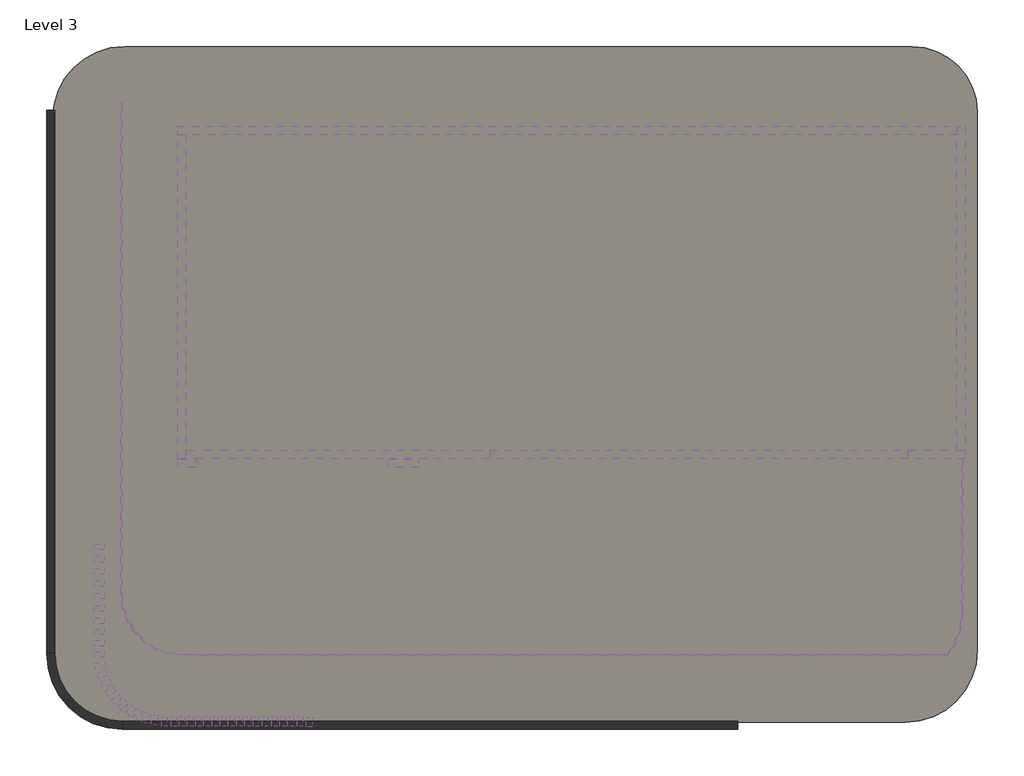
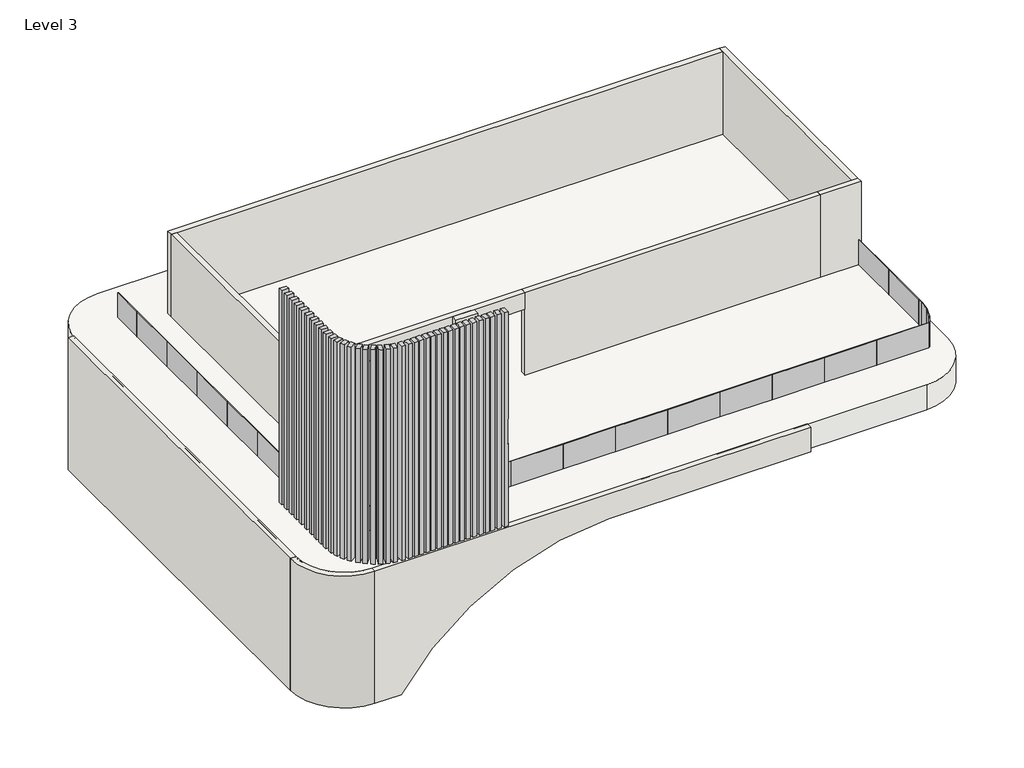
# One storey: 38 columns, 31 plates, 11 walls, 1 slab.
"""IFC4 building model written with IfcOpenShell, lengths in millimetres."""

from ifc_helpers import new_model, si_unit, point, frame, frame_2d, origin, place, context, project, spatial, polyline, circle_curve, trimmed, segment, composite_curve, outline, extrude, faceted_brep, transform, mapped, element, save
from components import wood_timber_column_6_x_10_a3b0a8a3, system_panel_glazed_95be5de7, system_panel_glazed_8df4d628, system_panel_glazed_8746fe8c, system_panel_glazed_e5de8428, system_panel_glazed_70ef586e, system_panel_glazed_2e848b93, system_panel_glazed_d6f392a9, system_panel_glazed_76d2efde, system_panel_glazed_ca107f82, system_panel_glazed_2060cbb7, system_panel_glazed_2c748f7c

model = new_model("IFC4")

# Units and contexts
model_context = context("Model", 3, world=origin())
ifc_project = project(units=[si_unit("LENGTHUNIT", "METRE", prefix="MILLI")], contexts=[model_context])

# Site, building, storey
site = spatial("IfcSite", under=ifc_project)
building = spatial("IfcBuilding", under=site)
storey = spatial("IfcBuildingStorey", under=building, Name="Level 3", Elevation=6096.0)

# Columns
placement = place(None, origin())
element("IfcColumn", 1, ObjectType="Wood Timber Column : 6 x 10", at=placement, inside=storey, context=model_context, shape_type="Brep", body=[
    faceted_brep([(-12385.9213551, -2400.8102607, 7931.15), (-12525.6213551, -2400.8102607, 7931.15), (-12525.6213551, -2159.5102607, 7931.15), (-12385.9213551, -2159.5102607, 7931.15), (-12385.9213551, -2400.8102607, 10979.15), (-12401.7963551, -2400.8102607, 10979.15), (-12401.7963551, -2400.8102607, 11893.55), (-12385.9213551, -2400.8102607, 11893.55), (-12385.9213551, -2400.8102607, 15855.95), (-12525.6213551, -2400.8102607, 15855.95), (-12525.6213551, -2159.5102607, 15855.95), (-12385.9213551, -2159.5102607, 15855.95), (-12385.9213551, -2284.9227607, 11893.55), (-12385.9213551, -2284.9227607, 10979.15), (-12401.7963551, -2284.9227607, 11893.55), (-12401.7963551, -2284.9227607, 10979.15)], [[[0, 1, 2, 3]], [[1, 0, 4, 5, 6, 7, 8, 9]], [[2, 1, 9, 10]], [[3, 2, 10, 11]], [[0, 3, 11, 8, 7, 12, 13, 4]], [[9, 8, 11, 10]], [[14, 15, 13, 12]], [[14, 12, 7, 6]], [[15, 14, 6, 5]], [[13, 15, 5, 4]]]),
])
wood_timber_column_6_x_10_shape = wood_timber_column_6_x_10_a3b0a8a3(model_context)
element("IfcColumn", 2, ObjectType="Wood Timber Column : 6 x 10", at=placement, inside=storey, context=model_context, shape_type="MappedRepresentation", body=[
    mapped(wood_timber_column_6_x_10_shape, transform((-12684.3713551, -2267.4602607, 0.0), x_axis=(1.0, 0.0, 0.0), y_axis=(0.0, 1.0, 0.0), z_axis=(0.0, 0.0, 1.0))),
])
element("IfcColumn", 3, ObjectType="Wood Timber Column : 6 x 10", at=placement, inside=storey, context=model_context, shape_type="MappedRepresentation", body=[
    mapped(wood_timber_column_6_x_10_shape, transform((-12912.9713551, -2267.4602607, 0.0), x_axis=(1.0, 0.0, 0.0), y_axis=(0.0, 1.0, 0.0), z_axis=(0.0, 0.0, 1.0))),
])
element("IfcColumn", 4, ObjectType="Wood Timber Column : 6 x 10", at=placement, inside=storey, context=model_context, shape_type="MappedRepresentation", body=[
    mapped(wood_timber_column_6_x_10_shape, transform((-13116.1713551, -2267.4602607, 0.0), x_axis=(1.0, 0.0, 0.0), y_axis=(0.0, 1.0, 0.0), z_axis=(0.0, 0.0, 1.0))),
])
element("IfcColumn", 5, ObjectType="Wood Timber Column : 6 x 10", at=placement, inside=storey, context=model_context, shape_type="MappedRepresentation", body=[
    mapped(wood_timber_column_6_x_10_shape, transform((-13319.3713551, -2267.4602607, 0.0), x_axis=(1.0, 0.0, 0.0), y_axis=(0.0, 1.0, 0.0), z_axis=(0.0, 0.0, 1.0))),
])
element("IfcColumn", 6, ObjectType="Wood Timber Column : 6 x 10", at=placement, inside=storey, context=model_context, shape_type="MappedRepresentation", body=[
    mapped(wood_timber_column_6_x_10_shape, transform((-13547.9713551, -2267.4602607, 0.0), x_axis=(1.0, 0.0, 0.0), y_axis=(0.0, 1.0, 0.0), z_axis=(0.0, 0.0, 1.0))),
])
element("IfcColumn", 7, ObjectType="Wood Timber Column : 6 x 10", at=placement, inside=storey, context=model_context, shape_type="MappedRepresentation", body=[
    mapped(wood_timber_column_6_x_10_shape, transform((-13776.5713551, -2267.4602607, 0.0), x_axis=(1.0, 0.0, 0.0), y_axis=(0.0, 1.0, 0.0), z_axis=(0.0, 0.0, 1.0))),
])
element("IfcColumn", 8, ObjectType="Wood Timber Column : 6 x 10", at=placement, inside=storey, context=model_context, shape_type="MappedRepresentation", body=[
    mapped(wood_timber_column_6_x_10_shape, transform((-13979.7713551, -2267.4602607, 0.0), x_axis=(1.0, 0.0, 0.0), y_axis=(0.0, 1.0, 0.0), z_axis=(0.0, 0.0, 1.0))),
])
element("IfcColumn", 9, ObjectType="Wood Timber Column : 6 x 10", at=placement, inside=storey, context=model_context, shape_type="MappedRepresentation", body=[
    mapped(wood_timber_column_6_x_10_shape, transform((-14182.9713551, -2267.4602607, 0.0), x_axis=(1.0, 0.0, 0.0), y_axis=(0.0, 1.0, 0.0), z_axis=(0.0, 0.0, 1.0))),
])
element("IfcColumn", 10, ObjectType="Wood Timber Column : 6 x 10", at=placement, inside=storey, context=model_context, shape_type="MappedRepresentation", body=[
    mapped(wood_timber_column_6_x_10_shape, transform((-14386.1713551, -2267.4602607, 0.0), x_axis=(1.0, 0.0, 0.0), y_axis=(0.0, 1.0, 0.0), z_axis=(0.0, 0.0, 1.0))),
])
element("IfcColumn", 11, ObjectType="Wood Timber Column : 6 x 10", at=placement, inside=storey, context=model_context, shape_type="MappedRepresentation", body=[
    mapped(wood_timber_column_6_x_10_shape, transform((-14589.3713551, -2267.4602607, 0.0), x_axis=(1.0, 0.0, 0.0), y_axis=(0.0, 1.0, 0.0), z_axis=(0.0, 0.0, 1.0))),
])
element("IfcColumn", 12, ObjectType="Wood Timber Column : 6 x 10", at=placement, inside=storey, context=model_context, shape_type="MappedRepresentation", body=[
    mapped(wood_timber_column_6_x_10_shape, transform((-14792.5713551, -2267.4602607, 0.0), x_axis=(1.0, 0.0, 0.0), y_axis=(0.0, 1.0, 0.0), z_axis=(0.0, 0.0, 1.0))),
])
element("IfcColumn", 13, ObjectType="Wood Timber Column : 6 x 10", at=placement, inside=storey, context=model_context, shape_type="MappedRepresentation", body=[
    mapped(wood_timber_column_6_x_10_shape, transform((-14995.7713551, -2267.4602607, 0.0), x_axis=(1.0, 0.0, 0.0), y_axis=(0.0, 1.0, 0.0), z_axis=(0.0, 0.0, 1.0))),
])
element("IfcColumn", 14, ObjectType="Wood Timber Column : 6 x 10", at=placement, inside=storey, context=model_context, shape_type="MappedRepresentation", body=[
    mapped(wood_timber_column_6_x_10_shape, transform((-15198.9713551, -2267.4602607, 0.0), x_axis=(1.0, 0.0, 0.0), y_axis=(0.0, 1.0, 0.0), z_axis=(0.0, 0.0, 1.0))),
])
element("IfcColumn", 15, ObjectType="Wood Timber Column : 6 x 10", at=placement, inside=storey, context=model_context, shape_type="MappedRepresentation", body=[
    mapped(wood_timber_column_6_x_10_shape, transform((-15402.1713551, -2267.4602607, 0.0), x_axis=(1.0, 0.0, 0.0), y_axis=(0.0, 1.0, 0.0), z_axis=(0.0, 0.0, 1.0))),
])
element("IfcColumn", 16, ObjectType="Wood Timber Column : 6 x 10", at=placement, inside=storey, context=model_context, shape_type="MappedRepresentation", body=[
    mapped(wood_timber_column_6_x_10_shape, transform((-15605.3713551, -2267.4602607, 0.0), x_axis=(1.0, 0.0, 0.0), y_axis=(0.0, 1.0, 0.0), z_axis=(0.0, 0.0, 1.0))),
])
element("IfcColumn", 17, ObjectType="Wood Timber Column : 6 x 10", at=placement, inside=storey, context=model_context, shape_type="MappedRepresentation", body=[
    mapped(wood_timber_column_6_x_10_shape, transform((-15808.5713551, -2267.4602607, 0.0), x_axis=(1.0, 0.0, 0.0), y_axis=(0.0, 1.0, 0.0), z_axis=(0.0, 0.0, 1.0))),
])
element("IfcColumn", 18, ObjectType="Wood Timber Column : 6 x 10", at=placement, inside=storey, context=model_context, shape_type="MappedRepresentation", body=[
    mapped(wood_timber_column_6_x_10_shape, transform((-16043.6573637, -2267.4602607, 0.0), x_axis=(1.0, 0.0, 0.0), y_axis=(0.0, 1.0, 0.0), z_axis=(0.0, 0.0, 1.0))),
])
element("IfcColumn", 19, ObjectType="Wood Timber Column : 6 x 10", at=placement, inside=storey, context=model_context, shape_type="MappedRepresentation", body=[
    mapped(wood_timber_column_6_x_10_shape, transform((-16291.3073637, -2235.7102607, 0.0), x_axis=(0.9848077530122059, -0.17364817766694274, 0.0), y_axis=(0.17364817766694274, 0.9848077530122059, 0.0), z_axis=(0.0, 0.0, 1.0))),
])
element("IfcColumn", 20, ObjectType="Wood Timber Column : 6 x 10", at=placement, inside=storey, context=model_context, shape_type="MappedRepresentation", body=[
    mapped(wood_timber_column_6_x_10_shape, transform((-16494.5073637, -2178.5602607, 0.0), x_axis=(0.9396926207859039, -0.3420201433256814, 0.0), y_axis=(0.3420201433256814, 0.9396926207859039, 0.0), z_axis=(0.0, 0.0, 1.0))),
])
element("IfcColumn", 21, ObjectType="Wood Timber Column : 6 x 10", at=placement, inside=storey, context=model_context, shape_type="MappedRepresentation", body=[
    mapped(wood_timber_column_6_x_10_shape, transform((-16697.7073637, -2096.0102607, 0.0), x_axis=(0.9131152763933471, -0.4077014741414377, 0.0), y_axis=(0.4077014741414377, 0.9131152763933471, 0.0), z_axis=(0.0, 0.0, 1.0))),
])
element("IfcColumn", 22, ObjectType="Wood Timber Column : 6 x 10", at=placement, inside=storey, context=model_context, shape_type="MappedRepresentation", body=[
    mapped(wood_timber_column_6_x_10_shape, transform((-16881.8573637, -2000.7602607, 0.0), x_axis=(0.8386705679454172, -0.5446390350150377, 0.0), y_axis=(0.5446390350150377, 0.8386705679454172, 0.0), z_axis=(0.0, 0.0, 1.0))),
])
element("IfcColumn", 23, ObjectType="Wood Timber Column : 6 x 10", at=placement, inside=storey, context=model_context, shape_type="MappedRepresentation", body=[
    mapped(wood_timber_column_6_x_10_shape, transform((-17066.0073637, -1867.4102607, 0.0), x_axis=(0.761929669986281, -0.6476597702456106, 0.0), y_axis=(0.6476597702456106, 0.761929669986281, 0.0), z_axis=(0.0, 0.0, 1.0))),
])
element("IfcColumn", 24, ObjectType="Wood Timber Column : 6 x 10", at=placement, inside=storey, context=model_context, shape_type="MappedRepresentation", body=[
    mapped(wood_timber_column_6_x_10_shape, transform((-17221.6504261, -1720.1154413, 0.0), x_axis=(0.7071067811865404, -0.7071067811865548, 0.0), y_axis=(0.7071067811865548, 0.7071067811865404, 0.0), z_axis=(0.0, 0.0, 1.0))),
])
element("IfcColumn", 25, ObjectType="Wood Timber Column : 6 x 10", at=placement, inside=storey, context=model_context, shape_type="MappedRepresentation", body=[
    mapped(wood_timber_column_6_x_10_shape, transform((-17380.4004261, -1524.5102607, 0.0), x_axis=(-0.573576436351034, 0.8191520442890003, 0.0), y_axis=(-0.8191520442890003, -0.573576436351034, 0.0), z_axis=(0.0, 0.0, 1.0))),
])
element("IfcColumn", 26, ObjectType="Wood Timber Column : 6 x 10", at=placement, inside=storey, context=model_context, shape_type="MappedRepresentation", body=[
    mapped(wood_timber_column_6_x_10_shape, transform((-17494.7004261, -1321.3102607, 0.0), x_axis=(0.42261826174068956, -0.9063077870366546, 0.0), y_axis=(0.9063077870366546, 0.42261826174068956, 0.0), z_axis=(0.0, 0.0, 1.0))),
])
element("IfcColumn", 27, ObjectType="Wood Timber Column : 6 x 10", at=placement, inside=storey, context=model_context, shape_type="MappedRepresentation", body=[
    mapped(wood_timber_column_6_x_10_shape, transform((-17583.6004261, -1106.3247114, 0.0), x_axis=(0.32556815445714654, -0.9455185755993203, 0.0), y_axis=(0.9455185755993203, 0.32556815445714654, 0.0), z_axis=(0.0, 0.0, 1.0))),
])
element("IfcColumn", 28, ObjectType="Wood Timber Column : 6 x 10", at=placement, inside=storey, context=model_context, shape_type="MappedRepresentation", body=[
    mapped(wood_timber_column_6_x_10_shape, transform((-17634.4004261, -881.9746594, 0.0), x_axis=(0.1391731009600554, -0.9902680687415719, 0.0), y_axis=(0.9902680687415719, 0.1391731009600554, 0.0), z_axis=(0.0, 0.0, 1.0))),
])
element("IfcColumn", 29, ObjectType="Wood Timber Column : 6 x 10", at=placement, inside=storey, context=model_context, shape_type="MappedRepresentation", body=[
    mapped(wood_timber_column_6_x_10_shape, transform((-17659.8004261, -610.1102607, 0.0), x_axis=(0.0, -1.0, 0.0), y_axis=(1.0, 0.0, 0.0), z_axis=(0.0, 0.0, 1.0))),
])
element("IfcColumn", 30, ObjectType="Wood Timber Column : 6 x 10", at=placement, inside=storey, context=model_context, shape_type="MappedRepresentation", body=[
    mapped(wood_timber_column_6_x_10_shape, transform((-17659.8004261, -330.7102607, 0.0), x_axis=(0.0, -1.0, 0.0), y_axis=(1.0, 0.0, 0.0), z_axis=(0.0, 0.0, 1.0))),
])
element("IfcColumn", 31, ObjectType="Wood Timber Column : 6 x 10", at=placement, inside=storey, context=model_context, shape_type="MappedRepresentation", body=[
    mapped(wood_timber_column_6_x_10_shape, transform((-17659.8004261, -51.3102607, 0.0), x_axis=(0.0, -1.0, 0.0), y_axis=(1.0, 0.0, 0.0), z_axis=(0.0, 0.0, 1.0))),
])
element("IfcColumn", 32, ObjectType="Wood Timber Column : 6 x 10", at=placement, inside=storey, context=model_context, shape_type="MappedRepresentation", body=[
    mapped(wood_timber_column_6_x_10_shape, transform((-17659.8004261, 228.0897393, 0.0), x_axis=(0.0, -1.0, 0.0), y_axis=(1.0, 0.0, 0.0), z_axis=(0.0, 0.0, 1.0))),
])
element("IfcColumn", 33, ObjectType="Wood Timber Column : 6 x 10", at=placement, inside=storey, context=model_context, shape_type="MappedRepresentation", body=[
    mapped(wood_timber_column_6_x_10_shape, transform((-17659.8004261, 532.8897393, 0.0), x_axis=(0.0, -1.0, 0.0), y_axis=(1.0, 0.0, 0.0), z_axis=(0.0, 0.0, 1.0))),
])
element("IfcColumn", 34, ObjectType="Wood Timber Column : 6 x 10", at=placement, inside=storey, context=model_context, shape_type="MappedRepresentation", body=[
    mapped(wood_timber_column_6_x_10_shape, transform((-17659.8004261, 837.6897393, 0.0), x_axis=(0.0, -1.0, 0.0), y_axis=(1.0, 0.0, 0.0), z_axis=(0.0, 0.0, 1.0))),
])
element("IfcColumn", 35, ObjectType="Wood Timber Column : 6 x 10", at=placement, inside=storey, context=model_context, shape_type="MappedRepresentation", body=[
    mapped(wood_timber_column_6_x_10_shape, transform((-17659.8004261, 1142.4897393, 0.0), x_axis=(0.0, -1.0, 0.0), y_axis=(1.0, 0.0, 0.0), z_axis=(0.0, 0.0, 1.0))),
])
element("IfcColumn", 36, ObjectType="Wood Timber Column : 6 x 10", at=placement, inside=storey, context=model_context, shape_type="MappedRepresentation", body=[
    mapped(wood_timber_column_6_x_10_shape, transform((-17659.8004261, 1447.2897393, 0.0), x_axis=(0.0, -1.0, 0.0), y_axis=(1.0, 0.0, 0.0), z_axis=(0.0, 0.0, 1.0))),
])
element("IfcColumn", 37, ObjectType="Wood Timber Column : 6 x 10", at=placement, inside=storey, context=model_context, shape_type="MappedRepresentation", body=[
    mapped(wood_timber_column_6_x_10_shape, transform((-17659.8004261, 1752.0897393, 0.0), x_axis=(0.0, -1.0, 0.0), y_axis=(1.0, 0.0, 0.0), z_axis=(0.0, 0.0, 1.0))),
])
element("IfcColumn", 38, ObjectType="Wood Timber Column : 6 x 10", at=placement, inside=storey, context=model_context, shape_type="MappedRepresentation", body=[
    mapped(wood_timber_column_6_x_10_shape, transform((-17659.8004261, 2056.8897393, 0.0), x_axis=(0.0, -1.0, 0.0), y_axis=(1.0, 0.0, 0.0), z_axis=(0.0, 0.0, 1.0))),
])

# Plates
system_panel_glazed_shape = system_panel_glazed_95be5de7(model_context)
element("IfcPlate", 39, ObjectType="System Panel : Glazed", at=placement, inside=storey, context=model_context, shape_type="MappedRepresentation", body=[
    mapped(system_panel_glazed_shape, transform((3693.0466756, 3328.5792748, 7931.15), x_axis=(0.0, -1.0, 0.0), y_axis=(1.0, 0.0, 0.0), z_axis=(0.0, 0.0, 1.0))),
])
element("IfcPlate", 40, ObjectType="System Panel : Glazed", at=placement, inside=storey, context=model_context, shape_type="MappedRepresentation", body=[
    mapped(system_panel_glazed_shape, transform((3693.0466756, 1499.7792748, 7931.15), x_axis=(0.0, -1.0, 0.0), y_axis=(1.0, 0.0, 0.0), z_axis=(0.0, 0.0, 1.0))),
])
element("IfcPlate", 41, ObjectType="System Panel : Glazed", at=placement, inside=storey, context=model_context, shape_type="MappedRepresentation", body=[
    mapped(system_panel_glazed_shape, transform((2445.8413412, -580.0497962, 7931.15), x_axis=(-1.0, 0.0, 0.0), y_axis=(0.0, -1.0, 0.0), z_axis=(0.0, 0.0, 1.0))),
])
element("IfcPlate", 42, ObjectType="System Panel : Glazed", at=placement, inside=storey, context=model_context, shape_type="MappedRepresentation", body=[
    mapped(system_panel_glazed_shape, transform((617.0413412, -580.0497962, 7931.15), x_axis=(-1.0, 0.0, 0.0), y_axis=(0.0, -1.0, 0.0), z_axis=(0.0, 0.0, 1.0))),
])
element("IfcPlate", 43, ObjectType="System Panel : Glazed", at=placement, inside=storey, context=model_context, shape_type="MappedRepresentation", body=[
    mapped(system_panel_glazed_shape, transform((-1211.7586588, -580.0497962, 7931.15), x_axis=(-1.0, 0.0, 0.0), y_axis=(0.0, -1.0, 0.0), z_axis=(0.0, 0.0, 1.0))),
])
element("IfcPlate", 44, ObjectType="System Panel : Glazed", at=placement, inside=storey, context=model_context, shape_type="MappedRepresentation", body=[
    mapped(system_panel_glazed_shape, transform((-3040.5586588, -580.0497962, 7931.15), x_axis=(-1.0, 0.0, 0.0), y_axis=(0.0, -1.0, 0.0), z_axis=(0.0, 0.0, 1.0))),
])
element("IfcPlate", 45, ObjectType="System Panel : Glazed", at=placement, inside=storey, context=model_context, shape_type="MappedRepresentation", body=[
    mapped(system_panel_glazed_shape, transform((-4869.3586588, -580.0497962, 7931.15), x_axis=(-1.0, 0.0, 0.0), y_axis=(0.0, -1.0, 0.0), z_axis=(0.0, 0.0, 1.0))),
])
element("IfcPlate", 46, ObjectType="System Panel : Glazed", at=placement, inside=storey, context=model_context, shape_type="MappedRepresentation", body=[
    mapped(system_panel_glazed_shape, transform((-6698.1586588, -580.0497962, 7931.15), x_axis=(-1.0, 0.0, 0.0), y_axis=(0.0, -1.0, 0.0), z_axis=(0.0, 0.0, 1.0))),
])
element("IfcPlate", 47, ObjectType="System Panel : Glazed", at=placement, inside=storey, context=model_context, shape_type="MappedRepresentation", body=[
    mapped(system_panel_glazed_shape, transform((-8526.9586588, -580.0497962, 7931.15), x_axis=(-1.0, 0.0, 0.0), y_axis=(0.0, -1.0, 0.0), z_axis=(0.0, 0.0, 1.0))),
])
element("IfcPlate", 48, ObjectType="System Panel : Glazed", at=placement, inside=storey, context=model_context, shape_type="MappedRepresentation", body=[
    mapped(system_panel_glazed_shape, transform((-17086.678953, 1829.8432662, 7931.15), x_axis=(0.0, 1.0, 0.0), y_axis=(-1.0, 0.0, 0.0), z_axis=(0.0, 0.0, 1.0))),
])
element("IfcPlate", 49, ObjectType="System Panel : Glazed", at=placement, inside=storey, context=model_context, shape_type="MappedRepresentation", body=[
    mapped(system_panel_glazed_shape, transform((-17086.678953, 3658.6432662, 7931.15), x_axis=(0.0, 1.0, 0.0), y_axis=(-1.0, 0.0, 0.0), z_axis=(0.0, 0.0, 1.0))),
])
element("IfcPlate", 50, ObjectType="System Panel : Glazed", at=placement, inside=storey, context=model_context, shape_type="MappedRepresentation", body=[
    mapped(system_panel_glazed_shape, transform((-10355.7586588, -580.0497962, 7931.15), x_axis=(-1.0, 0.0, 0.0), y_axis=(0.0, -1.0, 0.0), z_axis=(0.0, 0.0, 1.0))),
])
element("IfcPlate", 51, ObjectType="System Panel : Glazed", at=placement, inside=storey, context=model_context, shape_type="MappedRepresentation", body=[
    mapped(system_panel_glazed_shape, transform((-12184.5586588, -580.0497962, 7931.15), x_axis=(-1.0, 0.0, 0.0), y_axis=(0.0, -1.0, 0.0), z_axis=(0.0, 0.0, 1.0))),
])
element("IfcPlate", 52, ObjectType="System Panel : Glazed", at=placement, inside=storey, context=model_context, shape_type="MappedRepresentation", body=[
    mapped(system_panel_glazed_shape, transform((-14013.3586588, -580.0497962, 7931.15), x_axis=(-1.0, 0.0, 0.0), y_axis=(0.0, -1.0, 0.0), z_axis=(0.0, 0.0, 1.0))),
])
element("IfcPlate", 53, ObjectType="System Panel : Glazed", at=placement, inside=storey, context=model_context, shape_type="MappedRepresentation", body=[
    mapped(system_panel_glazed_shape, transform((-17086.678953, 5487.4432662, 7931.15), x_axis=(0.0, 1.0, 0.0), y_axis=(-1.0, 0.0, 0.0), z_axis=(0.0, 0.0, 1.0))),
])
element("IfcPlate", 54, ObjectType="System Panel : Glazed", at=placement, inside=storey, context=model_context, shape_type="MappedRepresentation", body=[
    mapped(system_panel_glazed_shape, transform((-17086.678953, 7316.2432662, 7931.15), x_axis=(0.0, 1.0, 0.0), y_axis=(-1.0, 0.0, 0.0), z_axis=(0.0, 0.0, 1.0))),
])
element("IfcPlate", 55, ObjectType="System Panel : Glazed", at=placement, inside=storey, context=model_context, shape_type="MappedRepresentation", body=[
    mapped(system_panel_glazed_shape, transform((-17086.678953, 9145.0432662, 7931.15), x_axis=(0.0, 1.0, 0.0), y_axis=(-1.0, 0.0, 0.0), z_axis=(0.0, 0.0, 1.0))),
])
element("IfcPlate", 56, ObjectType="System Panel : Glazed", at=placement, inside=storey, context=model_context, shape_type="MappedRepresentation", body=[
    mapped(system_panel_glazed_shape, transform((-17086.678953, 10973.8432662, 7931.15), x_axis=(0.0, 1.0, 0.0), y_axis=(-1.0, 0.0, 0.0), z_axis=(0.0, 0.0, 1.0))),
])
system_panel_glazed_2_shape = system_panel_glazed_8df4d628(model_context)
element("IfcPlate", 57, ObjectType="System Panel : Glazed", at=placement, inside=storey, context=model_context, shape_type="MappedRepresentation", body=[
    mapped(system_panel_glazed_2_shape, transform((3693.0466756, 509.1792748, 7931.15), x_axis=(0.0, -1.0, 0.0), y_axis=(1.0, 0.0, 0.0), z_axis=(0.0, 0.0, 1.0))),
])
system_panel_glazed_3_shape = system_panel_glazed_8746fe8c(model_context)
element("IfcPlate", 58, ObjectType="System Panel : Glazed", at=placement, inside=storey, context=model_context, shape_type="MappedRepresentation", body=[
    mapped(system_panel_glazed_3_shape, transform((-17062.4907484, 726.7948552, 7931.15), x_axis=(-0.12717730440498626, 0.9918799994174101, 0.0), y_axis=(-0.9918799994174101, -0.12717730440498626, 0.0), z_axis=(0.0, 0.0, 1.0))),
])
system_panel_glazed_4_shape = system_panel_glazed_e5de8428(model_context)
element("IfcPlate", 59, ObjectType="System Panel : Glazed", at=placement, inside=storey, context=model_context, shape_type="MappedRepresentation", body=[
    mapped(system_panel_glazed_4_shape, transform((3671.4580572, 242.1617647, 7931.15), x_axis=(-0.11242030431559645, -0.9936607445087025, 0.0), y_axis=(0.9936607445087025, -0.11242030431559645, 0.0), z_axis=(0.0, 0.0, 1.0))),
])
element("IfcPlate", 60, ObjectType="System Panel : Glazed", at=placement, inside=storey, context=model_context, shape_type="MappedRepresentation", body=[
    mapped(system_panel_glazed_4_shape, transform((3586.1949598, -129.8268009, 7931.15), x_axis=(-0.331577695656461, -0.9434279154991925, 0.0), y_axis=(0.9434279154991925, -0.331577695656461, 0.0), z_axis=(0.0, 0.0, 1.0))),
])
system_panel_glazed_5_shape = system_panel_glazed_70ef586e(model_context)
element("IfcPlate", 61, ObjectType="System Panel : Glazed", at=placement, inside=storey, context=model_context, shape_type="MappedRepresentation", body=[
    mapped(system_panel_glazed_5_shape, transform((-16977.3211317, 380.2162823, 7931.15), x_axis=(-0.3602087986279214, 0.9328717068230924, 0.0), y_axis=(-0.9328717068230924, -0.3602087986279214, 0.0), z_axis=(0.0, 0.0, 1.0))),
])
system_panel_glazed_6_shape = system_panel_glazed_2e848b93(model_context)
element("IfcPlate", 62, ObjectType="System Panel : Glazed", at=placement, inside=storey, context=model_context, shape_type="MappedRepresentation", body=[
    mapped(system_panel_glazed_6_shape, transform((-16812.8134084, 72.2891221, 7931.15), x_axis=(-0.5680307758785693, 0.8230073132450225, 0.0), y_axis=(-0.8230073132450225, -0.5680307758785693, 0.0), z_axis=(0.0, 0.0, 1.0))),
])
system_panel_glazed_7_shape = system_panel_glazed_d6f392a9(model_context)
element("IfcPlate", 63, ObjectType="System Panel : Glazed", at=placement, inside=storey, context=model_context, shape_type="MappedRepresentation", body=[
    mapped(system_panel_glazed_7_shape, transform((-16593.8266334, -183.0896648, 7931.15), x_axis=(-0.7386085467399861, 0.6741345671916296, 0.0), y_axis=(-0.6741345671916296, -0.7386085467399861, 0.0), z_axis=(0.0, 0.0, 1.0))),
])
system_panel_glazed_8_shape = system_panel_glazed_76d2efde(model_context)
element("IfcPlate", 64, ObjectType="System Panel : Glazed", at=placement, inside=storey, context=model_context, shape_type="MappedRepresentation", body=[
    mapped(system_panel_glazed_8_shape, transform((-15748.2974005, -563.3578788, 7931.15), x_axis=(-0.994403599652405, 0.10564791052519472, 0.0), y_axis=(-0.10564791052519472, -0.994403599652405, 0.0), z_axis=(0.0, 0.0, 1.0))),
])
element("IfcPlate", 65, ObjectType="System Panel : Glazed", at=placement, inside=storey, context=model_context, shape_type="MappedRepresentation", body=[
    mapped(system_panel_glazed_8_shape, transform((-16341.9846616, -368.2381812, 7931.15), x_axis=(-0.8631975005225224, 0.5048663933078434, 0.0), y_axis=(-0.5048663933078434, -0.8631975005225224, 0.0), z_axis=(0.0, 0.0, 1.0))),
])
element("IfcPlate", 66, ObjectType="System Panel : Glazed", at=placement, inside=storey, context=model_context, shape_type="MappedRepresentation", body=[
    mapped(system_panel_glazed_8_shape, transform((-16055.5060319, -497.3354353, 7931.15), x_axis=(-0.950007532123609, 0.31222698299219753, 0.0), y_axis=(-0.31222698299219753, -0.950007532123609, 0.0), z_axis=(0.0, 0.0, 1.0))),
])
system_panel_glazed_9_shape = system_panel_glazed_ca107f82(model_context)
element("IfcPlate", 67, ObjectType="System Panel : Glazed", at=placement, inside=storey, context=model_context, shape_type="MappedRepresentation", body=[
    mapped(system_panel_glazed_9_shape, transform((3441.380911, -445.5238263, 7931.15), x_axis=(-0.5164788007382739, -0.8562999757024138, 0.0), y_axis=(0.8562999757024138, -0.5164788007382739, 0.0), z_axis=(0.0, 0.0, 1.0))),
])
system_panel_glazed_10_shape = system_panel_glazed_2060cbb7(model_context)
element("IfcPlate", 68, ObjectType="System Panel : Glazed", at=placement, inside=storey, context=model_context, shape_type="MappedRepresentation", body=[
    mapped(system_panel_glazed_10_shape, transform((-17086.678953, 12466.1612705, 7931.15), x_axis=(0.0, 1.0, 0.0), y_axis=(-1.0, 0.0, 0.0), z_axis=(0.0, 0.0, 1.0))),
])
system_panel_glazed_11_shape = system_panel_glazed_2c748f7c(model_context)
element("IfcPlate", 69, ObjectType="System Panel : Glazed", at=placement, inside=storey, context=model_context, shape_type="MappedRepresentation", body=[
    mapped(system_panel_glazed_11_shape, transform((-15259.4722747, -580.0497962, 7931.15), x_axis=(-1.0, 0.0, 0.0), y_axis=(0.0, -1.0, 0.0), z_axis=(0.0, 0.0, 1.0))),
])

# Slab
element("IfcSlab", 70, ObjectType="Generic - 3'", at=placement, inside=storey, context=model_context, shape_type="SweptSolid", body=[
    extrude(outline(composite_curve([segment(trimmed(circle_curve(frame_2d((2475.3420879, 12828.0432662)), 1625.6), [point((2475.3420879, 14453.6432662))], [point((4100.9420879, 12828.0432662))], False, "CARTESIAN"), True, "CONTINUOUS"), segment(polyline([(4100.9420879, 12828.0432662), (4100.9420879, -506.9567338)]), True, "CONTINUOUS"), segment(trimmed(circle_curve(frame_2d((2322.9420879, -506.9567338)), 1778.0), [point((4100.9420879, -506.9567338))], [point((2322.9420879, -2284.9567338))], False, "CARTESIAN"), True, "CONTINUOUS"), segment(polyline([(2322.9420879, -2284.9567338), (-17033.3533244, -2284.9567338)]), True, "CONTINUOUS"), segment(trimmed(circle_curve(frame_2d((-17033.3533244, -506.9567338)), 1778.0), [point((-17033.3533244, -2284.9567338))], [point((-18811.3533244, -506.9567338))], False, "CARTESIAN"), True, "CONTINUOUS"), segment(polyline([(-18811.3533244, -506.9567338), (-18811.3533244, 12675.6432662)]), True, "CONTINUOUS"), segment(trimmed(circle_curve(frame_2d((-17033.3533244, 12675.6432662)), 1778.0), [point((-18811.3533244, 12675.6432662))], [point((-17033.3533244, 14453.6432662))], False, "CARTESIAN"), True, "CONTINUOUS"), segment(polyline([(-17033.3533244, 14453.6432662), (2475.3420879, 14453.6432662)]), True, "CONTINUOUS")], self_intersect=False)), frame((0.0, 0.0, 7010.4), z_axis=(0.0, 0.0, 1.0), x_axis=(1.0, 0.0, 0.0)), (0.0, 0.0, 1.0), 914.4),
])

# Walls
element("IfcWall", 71, ObjectType="Generic - 8\" brown", at=placement, inside=storey, context=model_context, shape_type="SweptSolid", body=[
    extrude(outline(polyline([(-15255.3533244, 4027.0792748), (-15712.5533244, 4027.0792748), (-15712.5533244, 4230.2792748), (-15255.3533244, 4230.2792748), (-15255.3533244, 4027.0792748)])), frame((0.0, 0.0, 7931.15), z_axis=(0.0, 0.0, 1.0), x_axis=(1.0, 0.0, 0.0)), (0.0, 0.0, 1.0), 3048.0),
])
element("IfcWall", 72, ObjectType="Generic - 8\" brown", at=placement, inside=storey, context=model_context, shape_type="SweptSolid", body=[
    extrude(outline(polyline([(-9743.5533244, 4027.0792748), (-10505.5533244, 4027.0792748), (-10505.5533244, 4230.2792748), (-9743.5533244, 4230.2792748), (-9743.5533244, 4027.0792748)])), frame((0.0, 0.0, 7931.15), z_axis=(0.0, 0.0, 1.0), x_axis=(1.0, 0.0, 0.0)), (0.0, 0.0, 1.0), 3048.0),
])
element("IfcWall", 73, ObjectType="Generic - 8\" white wood", at=placement, inside=storey, context=model_context, shape_type="SweptSolid", body=[
    extrude(outline(polyline([(-18963.7533244, -583.1567338), (-18963.7533244, 12878.8432662), (-18760.5533244, 12878.8432662), (-18760.5533244, -583.1567338), (-18963.7533244, -583.1567338)])), frame((0.0, 0.0, 3048.0), z_axis=(0.0, 0.0, 1.0), x_axis=(1.0, 0.0, 0.0)), (0.0, 0.0, 1.0), 4876.8),
])
element("IfcWall", 74, ObjectType="Generic - 8\" white wood", at=placement, inside=storey, context=model_context, shape_type="SweptSolid", body=[
    extrude(outline(composite_curve([segment(polyline([(-17084.1533244, -2259.5567338), (-17084.1533244, -2462.7567338)]), True, "CONTINUOUS"), segment(trimmed(circle_curve(frame_2d((-17084.1533244, -583.1567338)), 1879.6), [point((-17084.1533244, -2462.7567338))], [point((-18963.7533244, -583.1567338))], False, "CARTESIAN"), True, "CONTINUOUS"), segment(polyline([(-18963.7533244, -583.1567338), (-18760.5533244, -583.1567338)]), True, "CONTINUOUS"), segment(trimmed(circle_curve(frame_2d((-17084.1533244, -583.1567338)), 1676.4), [point((-18760.5533244, -583.1567338))], [point((-17084.1533244, -2259.5567338))], True, "CARTESIAN"), True, "CONTINUOUS")], self_intersect=False)), frame((0.0, 0.0, 3048.0), z_axis=(0.0, 0.0, 1.0), x_axis=(1.0, 0.0, 0.0)), (0.0, 0.0, 1.0), 4876.8),
])
element("IfcWall", 75, ObjectType="Generic - 8\" white wood", at=placement, inside=storey, context=model_context, shape_type="SweptSolid", body=[
    extrude(outline(composite_curve([segment(polyline([(3048.0, -17084.1533244), (3048.0, -16169.7533244)]), True, "CONTINUOUS"), segment(trimmed(circle_curve(frame_2d((-1955.8, -8727.5533244)), 8967.9627162), [point((3048.0, -16169.7533244))], [point((7010.4, -8905.3533244))], True, "CARTESIAN"), True, "CONTINUOUS"), segment(polyline([(7010.4, -8905.3533244), (7010.4, -1837.8033244), (7924.8, -1837.8033244), (7924.8, -17084.1533244), (3048.0, -17084.1533244)]), True, "CONTINUOUS")], self_intersect=False)), frame((0.0, -2462.7567338, 0.0), z_axis=(0.0, 1.0, 0.0), x_axis=(0.0, 0.0, 1.0)), (0.0, 0.0, 1.0), 203.2),
])
element("IfcWall", 76, ObjectType="Generic - 8\" wood", at=placement, inside=storey, context=model_context, shape_type="Brep", body=[
    faceted_brep([(-15712.5533244, 12269.3792748, 7931.15), (-15509.3533244, 12269.3792748, 7931.15), (3591.4466756, 12269.3792748, 7931.15), (3591.4466756, 12269.3792748, 10979.15), (-15509.3533244, 12269.3792748, 10979.15), (-15712.5533244, 12269.3792748, 10979.15), (-15712.5533244, 12472.5792748, 7931.15), (-15712.5533244, 12472.5792748, 10979.15), (3591.4466756, 12472.5792748, 10979.15), (3591.4466756, 12472.5792748, 7931.15)], [[[0, 1, 2, 3, 4, 5]], [[6, 7, 8, 9]], [[2, 1, 0, 6, 9]], [[5, 4, 3, 8, 7]], [[0, 5, 7, 6]], [[3, 2, 9, 8]]]),
])
element("IfcWall", 77, ObjectType="Generic - 8\" wood", at=placement, inside=storey, context=model_context, shape_type="Brep", body=[
    faceted_brep([(-15509.3533244, 4242.9792748, 7931.15), (-15509.3533244, 4446.1792748, 7931.15), (-15509.3533244, 12269.3792748, 7931.15), (-15509.3533244, 12269.3792748, 10979.15), (-15509.3533244, 4446.1792748, 10979.15), (-15509.3533244, 4242.9792748, 10979.15), (-15712.5533244, 4242.9792748, 7931.15), (-15712.5533244, 4242.9792748, 10979.15), (-15712.5533244, 12269.3792748, 10979.15), (-15712.5533244, 12269.3792748, 7931.15)], [[[0, 1, 2, 3, 4, 5]], [[6, 7, 8, 9]], [[2, 1, 0, 6, 9]], [[5, 4, 3, 8, 7]], [[0, 5, 7, 6]], [[3, 2, 9, 8]]]),
])
element("IfcWall", 78, ObjectType="Generic - 8\" wood", at=placement, inside=storey, context=model_context, shape_type="Brep", body=[
    faceted_brep([(3794.6466756, 4446.1792748, 7931.15), (3591.4466756, 4446.1792748, 7931.15), (2372.2466756, 4446.1792748, 7931.15), (2372.2466756, 4446.1792748, 10979.15), (3591.4466756, 4446.1792748, 10979.15), (3794.6466756, 4446.1792748, 10979.15), (3794.6466756, 4242.9792748, 7931.15), (3794.6466756, 4242.9792748, 10979.15), (2372.2466756, 4242.9792748, 10979.15), (2372.2466756, 4242.9792748, 7931.15)], [[[0, 1, 2, 3, 4, 5]], [[6, 7, 8, 9]], [[2, 1, 0, 6, 9]], [[3, 2, 9, 8]], [[5, 4, 3, 8, 7]], [[0, 5, 7, 6]]]),
])
element("IfcWall", 79, ObjectType="Generic - 8\" wood", at=placement, inside=storey, context=model_context, shape_type="Brep", body=[
    faceted_brep([(3591.4466756, 12472.5792748, 7931.15), (3591.4466756, 12269.3792748, 7931.15), (3591.4466756, 4446.1792748, 7931.15), (3591.4466756, 4446.1792748, 10979.15), (3591.4466756, 12269.3792748, 10979.15), (3591.4466756, 12472.5792748, 10979.15), (3794.6466756, 12472.5792748, 7931.15), (3794.6466756, 12472.5792748, 10979.15), (3794.6466756, 4446.1792748, 10979.15), (3794.6466756, 4446.1792748, 7931.15)], [[[0, 1, 2, 3, 4, 5]], [[6, 7, 8, 9]], [[2, 1, 0, 6, 9]], [[5, 4, 3, 8, 7]], [[0, 5, 7, 6]], [[3, 2, 9, 8]]]),
])
element("IfcWall", 80, ObjectType="Generic - 8\" wood", at=placement, inside=storey, context=model_context, shape_type="SweptSolid", body=[
    extrude(outline(polyline([(7931.15, -15509.3533244), (7931.15, -14243.2931037), (10369.55, -14243.2931037), (10369.55, -12109.6931037), (7931.15, -12109.6931037), (7931.15, -8802.0384076), (10369.55, -8802.0384076), (10369.55, -7965.5533244), (10979.15, -7965.5533244), (10979.15, -15509.3533244), (7931.15, -15509.3533244)])), frame((0.0, 4242.9792748, 0.0), z_axis=(0.0, 1.0, 0.0), x_axis=(0.0, 0.0, 1.0)), (0.0, 0.0, 1.0), 203.2),
])
element("IfcWall", 81, ObjectType="Generic - 8\" wood 2", at=placement, inside=storey, context=model_context, shape_type="SweptSolid", body=[
    extrude(outline(polyline([(-7965.5533244, 4446.1792748), (2372.2466756, 4446.1792748), (2372.2466756, 4242.9792748), (-7965.5533244, 4242.9792748), (-7965.5533244, 4446.1792748)])), frame((0.0, 0.0, 7931.15), z_axis=(0.0, 0.0, 1.0), x_axis=(1.0, 0.0, 0.0)), (0.0, 0.0, 1.0), 3048.0),
])

save(model, "model.ifc")

# Revit data of these elements
# Type "Wood Timber Column : 6 x 10"
#   Assembly Code = "B1010200"
#   Depth = 0' - 9 1/2"
#   Width = 0' - 5 1/2"
#   Material = Softwood, Lumber
# Type "System Panel : Glazed"
#   Construction Type Id = "GSP4R"
#   Analytic Construction = "1/8 in Pilkington single glazing"
#   Visual Light Transmittance = 0.9
#   Solar Heat Gain Coefficient = 0.86
#   Heat Transfer Coefficient (U) = 1.18115 BTU/(h·ft²·°F)
# Type "Generic - 3'"
#   Assembly Code = "B1010"
#   Function = 0
#   Layers, outside or top first: 3' - 0" "Cherry" (function 1)
# Type "Generic - 8\" brown"
#   Assembly Code = "B2010"
#   Layers, outside or top first: 0' - 8" "Door - Panel" (function 1)
# Type "Generic - 8\" white wood"
#   Assembly Code = "B2010"
#   Layers, outside or top first: 0' - 8" "Tile, Porcelain, 4in" (function 1)
# Type "Generic - 8\" wood"
#   Assembly Code = "B2010"
#   Layers, outside or top first: 0' - 8" "Cherry" (function 1)
# Type "Generic - 8\" wood 2"
#   Assembly Code = "B2010"
#   Layers, outside or top first: 0' - 8" "Concrete, Precast" (function 1)
# Element 1 (IfcColumn, "Wood Timber Column : 6 x 10")
#   Phase Created = New Construction
#   Materials on its faces: "Softwood, Lumber", "Tile, Porcelain, 4in"
# Elements 2, 3, 4, 5, 6, 7, 8, 9, 10, 11, 12, 13, 14, 15, 16, 17, 18, 19, 20, 21, 22, 23, 24, 25, 26, 27, 28, 29, 30, 31, 32, 33, 34, 35, 36, 37, 38 (IfcColumn, "Wood Timber Column : 6 x 10")
#   Phase Created = New Construction
#   Materials on its faces: "Softwood, Lumber"
# Elements 39, 40, 41, 42, 43, 44, 45, 46, 47, 48, 49, 50, 51, 52, 53, 54, 55, 56, 57, 58, 59, 60, 61, 62, 63, 64, 65, 66, 67, 68, 69 (IfcPlate, "System Panel : Glazed")
#   Phase Created = New Construction
#   Materials on its faces: "Glass"
# Element 70 (IfcSlab, "Generic - 3'")
#   Height Offset From Level = 6' - 0"
#   Phase Created = New Construction
#   Materials on its faces: "Cherry"
# Elements 71, 72 (IfcWall, "Generic - 8\" brown")
#   built-in parameter 1001111 = 6' - 0 1/4"
#   Top Offset = 0' - 0"
#   Base Offset = 6' - 0 1/4"
#   Unconnected Height = 10' - 0"
#   wall height = 10' - 0"
#   Phase Created = New Construction
#   Base Constraint = Level 3
#   Materials on its faces: "Door - Panel"
# Elements 73, 75 (IfcWall, "Generic - 8\" white wood")
#   built-in parameter 1001111 = -10' - 0"
#   Top Offset = 0' - 0"
#   Base Offset = -10' - 0"
#   Unconnected Height = 16' - 0"
#   wall height = 16' - 0"
#   Phase Created = New Construction
#   Base Constraint = Level 3
#   Materials on its faces: "Tile, Porcelain, 4in"
# Element 74 (IfcWall, "Generic - 8\" white wood")
#   built-in parameter 1001111 = -10' - 0"
#   Top Offset = 0' - 0"
#   Base Offset = -10' - 0"
#   Unconnected Height = 16' - 0"
#   wall height = 16' - 0"
#   Phase Created = New Construction
#   Materials on its faces: "Tile, Porcelain, 4in"
# Elements 76, 77, 78, 79, 80 (IfcWall, "Generic - 8\" wood")
#   built-in parameter 1001111 = 6' - 0 1/4"
#   Top Offset = 0' - 0"
#   Base Offset = 6' - 0 1/4"
#   Unconnected Height = 10' - 0"
#   wall height = 10' - 0"
#   Phase Created = New Construction
#   Base Constraint = Level 3
#   Materials on its faces: "Cherry"
# Element 81 (IfcWall, "Generic - 8\" wood 2")
#   built-in parameter 1001111 = 6' - 0 1/4"
#   Top Offset = 0' - 0"
#   Base Offset = 6' - 0 1/4"
#   Unconnected Height = 10' - 0"
#   wall height = 10' - 0"
#   Phase Created = New Construction
#   Base Constraint = Level 3
#   Materials on its faces: "Concrete, Precast"
# Materials
#   "Softwood, Lumber": class "Wood", colour RGB 223 192 134, transparency 0, Description = "Pinus Echinata", Cost = 0
#   "Cherry": class "Wood", colour RGB 238 208 179, transparency 0, Description = "Prunus Serotina", Cost = 0
#   "Door - Panel": class "Wood", colour RGB 210 159 95, transparency 0, Cost = 0
#   "Tile, Porcelain, 4in": class "Generic", colour RGB 89 87 158, transparency 0, Description = "Porcelain tile, 4\", white", Cost = 0
#   "Concrete, Precast": class "Concrete", colour RGB 198 187 187, transparency 0, Description = "Precast concrete", Cost = 0
#   "Glass": class "Glass", colour RGB 0 128 192, transparency 0.75, Description = "Soda Lime Glass", Cost = 0
